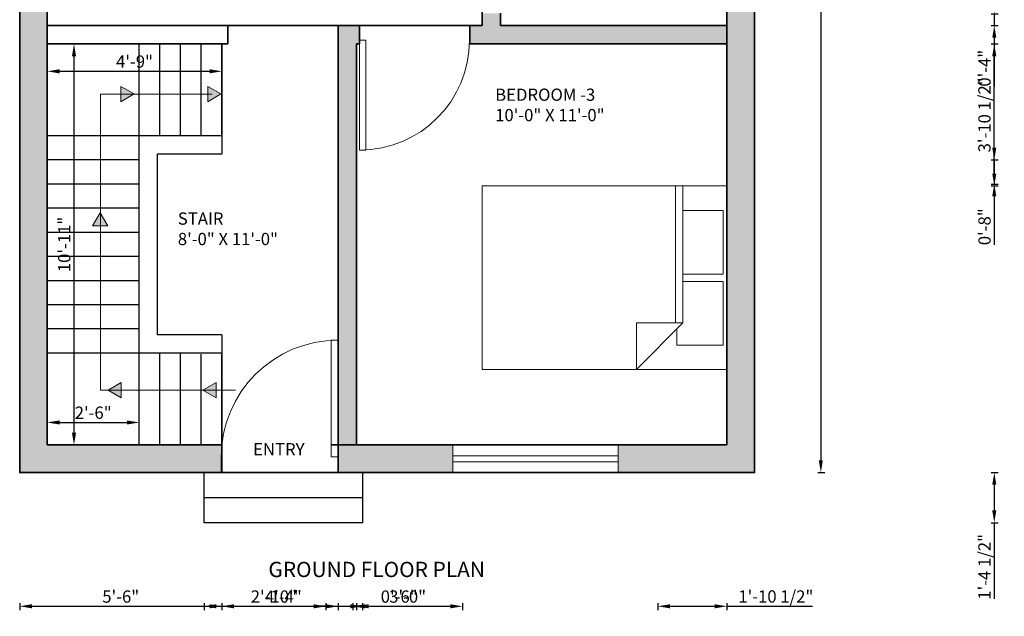
# Model space of a CAD drawing. Units: inches. Extents: x -35 to 322, y -513 to 50.
# Tile 1 of 3: x 1 to 322, y -513 to -318. Entities that reach past the tile are written whole.
import ezdxf

# ---------------------------------------------------------------- set-up
doc = ezdxf.new("R2010")
doc.units = ezdxf.units.IN
for name, color, linetype, lineweight in [('A-ANNO-DIMS', 2, 'Continuous', 18), ('A-ANNO-SYMB', 7, 'Continuous', 18), ('A-ANNO-TEXT', 7, 'Continuous', 25), ('A-AREA-IDEN', 7, 'Continuous', 18), ('A-DOOR', 4, 'Continuous', 18), ('A-FLOR-STRS', 7, 'Continuous', 25), ('A-FURN', 8, 'Continuous', 18), ('A-GLAZ', 6, 'Continuous', 18), ('A-WALL', 7, 'Continuous', 35), ('A-WALL-PATT', 251, 'Continuous', 13)]:
    doc.layers.add(name, color=color, linetype=linetype, lineweight=lineweight)
doc.styles.get("Standard").update_dxf_attribs({"font": 'arial.ttf'})
doc.dimstyles.new('ISO-25', dxfattribs={"dimtxt": 4, "dimasz": 4, "dimexe": 1.25, "dimexo": 0.625, "dimtad": 1, "dimlunit": 3, "dimtxsty": 'Standard', "dimcen": 2.5, "dimadec": 0, "dimazin": 0, "dimtfac": 1, "dimtmove": 0, "dimatfit": 3, "dimfxl": 1, "dimfxlon": 1, "dimarcsym": 0})

# ---------------------------------------------------------------- blocks, each defined once
blk = doc.blocks.new('*U4')
for p, q in [((0, 0), (0, -100)), ((750, 0), (750, -100))]:
    blk.add_line(p, q)
blk.add_lwpolyline([(0, 0), (0, 750), (43.75, 750), (43.75, 0)], close=True)
blk.add_arc((0, 0), 750, 0, 90)
blk = doc.blocks.new('Bed - Queen')
for p, q in [((0, -80.00003), (0, 0)), ((0, 0), (59.99999, 0)), ((59.99999, 0), (59.99999, -80.00003)), ((7.99999, -1.2), (28.79998, -1.2)), ((7.99999, -14.4), (7.99999, -1.2)), ((28.79998, -1.2), (28.79998, -14.4)), ((31.19999, -1.2), (51.99999, -1.2)), ((31.19999, -14.4), (31.19999, -1.2)), ((51.99999, -1.2), (51.99999, -16.4)), ((0, -14.4), (44.8, -14.4)), ((59.99999, -29.6), (44.8, -14.4)), ((44.8, -14.4), (44.8, -29.6)), ((44.8, -16.8), (0, -16.8)), ((51.99999, -16.4), (46.79936, -16.4)), ((44.8, -29.6), (59.99999, -29.6)), ((59.99999, -80.00003), (0, -80.00003))]:
    blk.add_line(p, q)
blk = doc.blocks.new('*D9')
at = {"layer": 'A-ANNO-DIMS', "color": 0, "lineweight": -2, "transparency": 16777216}
for p, q in [((9.64, -450.66), (9.64, -448.41)), ((13.64, -449.66), (35.64, -449.66)), ((39.64, -450.66), (39.64, -448.41))]:
    blk.add_line(p, q, dxfattribs=at)
at = {"layer": 'A-ANNO-DIMS', "color": 0, "transparency": 16777216}
for points in [[(13.64, -448.99), (13.64, -450.32), (9.64, -449.66)], [(35.64, -448.99), (35.64, -450.32), (39.64, -449.66)]]:
    blk.add_solid(points, dxfattribs=at)
at = {"layer": 'Defpoints', "color": 0, "transparency": 16777216}
for p in [(39.64, -449.66), (39.64, -455.32), (9.64, -457.01)]:
    blk.add_point(p, dxfattribs=at)
at = {"layer": 'A-ANNO-DIMS', "color": 0, "transparency": 16777216, "insert": (24.64, -446.99), "char_height": 4, "attachment_point": 5}
blk.add_mtext('2\'-6"', dxfattribs=at)
blk = doc.blocks.new('*D10')
at = {"layer": 'A-ANNO-DIMS', "color": 0, "lineweight": -2, "transparency": 16777216}
for p, q in [((17.38, -326.01), (19.63, -326.01)), ((18.38, -453.01), (18.38, -330.01)), ((17.38, -457.01), (19.63, -457.01))]:
    blk.add_line(p, q, dxfattribs=at)
at = {"layer": 'A-ANNO-DIMS', "color": 0, "transparency": 16777216}
for points in [[(17.71, -330.01), (19.04, -330.01), (18.38, -326.01)], [(17.71, -453.01), (19.04, -453.01), (18.38, -457.01)]]:
    blk.add_solid(points, dxfattribs=at)
at = {"layer": 'Defpoints', "color": 0, "transparency": 16777216}
for p in [(9.64, -326.01), (18.38, -326.01), (9.64, -457.01)]:
    blk.add_point(p, dxfattribs=at)
at = {"layer": 'A-ANNO-DIMS', "color": 0, "transparency": 16777216, "insert": (15.71, -391.51), "char_height": 4, "attachment_point": 5, "rotation": 90}
blk.add_mtext('10\'-11"', dxfattribs=at)
blk = doc.blocks.new('*D11')
at = {"layer": 'A-ANNO-DIMS', "color": 0, "lineweight": -2, "transparency": 16777216}
for p, q in [((9.64, -333.96), (9.64, -336.21)), ((66.64, -333.96), (66.64, -336.21)), ((13.64, -334.96), (62.64, -334.96))]:
    blk.add_line(p, q, dxfattribs=at)
at = {"layer": 'A-ANNO-DIMS', "color": 0, "transparency": 16777216}
for points in [[(13.64, -334.29), (13.64, -335.62), (9.64, -334.96)], [(62.64, -334.29), (62.64, -335.62), (66.64, -334.96)]]:
    blk.add_solid(points, dxfattribs=at)
at = {"layer": 'Defpoints', "color": 0, "transparency": 16777216}
for p in [(9.64, -326.01), (66.64, -326.01), (66.64, -334.96)]:
    blk.add_point(p, dxfattribs=at)
at = {"layer": 'A-ANNO-DIMS', "color": 0, "transparency": 16777216, "insert": (38.14, -332.29), "char_height": 4, "attachment_point": 5}
blk.add_mtext('4\'-9"', dxfattribs=at)
blk = doc.blocks.new('*D13')
at = {"layer": 'A-ANNO-DIMS', "color": 0, "lineweight": -2, "transparency": 16777216}
for p, q in [((261.29, 13.99), (263.54, 13.99)), ((262.29, 9.99), (262.29, -462.01)), ((261.29, -466.01), (263.54, -466.01))]:
    blk.add_line(p, q, dxfattribs=at)
at = {"layer": 'A-ANNO-DIMS', "color": 0, "transparency": 16777216}
for points in [[(261.62, 9.99), (262.95, 9.99), (262.29, 13.99)], [(261.62, -462.01), (262.95, -462.01), (262.29, -466.01)]]:
    blk.add_solid(points, dxfattribs=at)
at = {"layer": 'Defpoints', "color": 0, "transparency": 16777216}
for p in [(239.43, 13.99), (240.64, -466.01), (262.29, -466.01)]:
    blk.add_point(p, dxfattribs=at)
at = {"layer": 'A-ANNO-DIMS', "color": 0, "transparency": 16777216, "insert": (259.62, -226.01), "char_height": 4, "attachment_point": 5, "rotation": 90}
blk.add_mtext("40'", dxfattribs=at)
blk = doc.blocks.new('STAIR-DIRECTION-ARROW')
h = blk.add_hatch(color=256)
h.dxf.hatch_style = 1
h.paths.add_polyline_path([(0, 2.47), (4.31, 0), (4.31, 5)])
blk.add_lwpolyline([(4.31, 0), (4.31, 5), (0, 2.47)], close=True)
blk = doc.blocks.new('*D26')
at = {"layer": 'A-ANNO-DIMS', "color": 0, "lineweight": -2, "transparency": 16777216}
for p, q in [((100.64, -509.7), (96.64, -509.7)), ((104.64, -508.7), (104.64, -510.95)), ((104.64, -509.7), (110.64, -509.7)), ((110.64, -508.7), (110.64, -510.95)), ((114.64, -509.7), (130.52, -509.7))]:
    blk.add_line(p, q, dxfattribs=at)
at = {"layer": 'A-ANNO-DIMS', "color": 0, "transparency": 16777216}
for points in [[(100.64, -509.04), (100.64, -510.37), (104.64, -509.7)], [(114.64, -509.04), (114.64, -510.37), (110.64, -509.7)]]:
    blk.add_solid(points, dxfattribs=at)
at = {"layer": 'Defpoints', "color": 0, "transparency": 16777216}
for p in [(104.64, -77.01), (110.64, -83.01), (110.64, -509.7)]:
    blk.add_point(p, dxfattribs=at)
at = {"layer": 'A-ANNO-DIMS', "color": 0, "transparency": 16777216, "insert": (124.58, -507.04), "char_height": 4, "attachment_point": 5}
blk.add_mtext('0\'-6"', dxfattribs=at)
blk = doc.blocks.new('*D27')
at = {"layer": 'A-ANNO-DIMS', "color": 0, "lineweight": -2, "transparency": 16777216}
for p, q in [((60.84, -508.7), (60.84, -510.95)), ((64.84, -509.7), (108.62, -509.7)), ((112.62, -508.7), (112.62, -510.95))]:
    blk.add_line(p, q, dxfattribs=at)
at = {"layer": 'A-ANNO-DIMS', "color": 0, "transparency": 16777216}
for points in [[(64.84, -509.04), (64.84, -510.37), (60.84, -509.7)], [(108.62, -509.04), (108.62, -510.37), (112.62, -509.7)]]:
    blk.add_solid(points, dxfattribs=at)
at = {"layer": 'Defpoints', "color": 0, "transparency": 16777216}
for p in [(60.84, -482.4), (112.62, -482.4), (112.62, -509.7)]:
    blk.add_point(p, dxfattribs=at)
at = {"layer": 'A-ANNO-DIMS', "color": 0, "transparency": 16777216, "insert": (86.73, -507.08), "char_height": 4, "attachment_point": 5}
blk.add_mtext('4\'-4"', dxfattribs=at)
blk = doc.blocks.new('*D28')
at = {"layer": 'A-ANNO-DIMS', "color": 0, "lineweight": -2, "transparency": 16777216}
for p, q in [((317.94, -466.01), (320.19, -466.01)), ((318.94, -470.01), (318.94, -478.4)), ((317.94, -482.4), (320.19, -482.4)), ((318.94, -482.4), (318.94, -507.23))]:
    blk.add_line(p, q, dxfattribs=at)
at = {"layer": 'A-ANNO-DIMS', "color": 0, "transparency": 16777216}
for points in [[(318.27, -470.01), (319.6, -470.01), (318.94, -466.01)], [(318.27, -478.4), (319.6, -478.4), (318.94, -482.4)]]:
    blk.add_solid(points, dxfattribs=at)
at = {"layer": 'Defpoints', "color": 0, "transparency": 16777216}
for p in [(112.62, -466.01), (112.62, -482.4), (318.94, -482.4)]:
    blk.add_point(p, dxfattribs=at)
at = {"layer": 'A-ANNO-DIMS', "color": 0, "transparency": 16777216, "insert": (316.24, -496.82), "char_height": 4, "attachment_point": 5, "rotation": 90}
blk.add_mtext('1\'-4 1/2"', dxfattribs=at)
blk = doc.blocks.new('*D29')
at = {"layer": 'A-ANNO-DIMS', "color": 0, "lineweight": -2, "transparency": 16777216}
for p, q in [((66.64, 40.29), (66.64, 42.54)), ((104.64, 40.29), (104.64, 42.54)), ((70.64, 41.29), (100.64, 41.29))]:
    blk.add_line(p, q, dxfattribs=at)
at = {"layer": 'A-ANNO-DIMS', "color": 0, "transparency": 16777216}
for points in [[(70.64, 41.95), (70.64, 40.62), (66.64, 41.29)], [(100.64, 41.95), (100.64, 40.62), (104.64, 41.29)]]:
    blk.add_solid(points, dxfattribs=at)
at = {"layer": 'Defpoints', "color": 0, "transparency": 16777216}
for p in [(104.64, 41.29), (66.64, -466.01), (104.64, -466.01)]:
    blk.add_point(p, dxfattribs=at)
at = {"layer": 'A-ANNO-DIMS', "color": 0, "transparency": 16777216, "insert": (85.64, 43.96), "char_height": 4, "attachment_point": 5}
blk.add_mtext('3\'-2"', dxfattribs=at)
blk = doc.blocks.new('*D30')
at = {"layer": 'A-ANNO-DIMS', "color": 0, "lineweight": -2, "transparency": 16777216}
for p, q in [((0.64, -508.7), (0.64, -510.95)), ((4.64, -509.7), (62.64, -509.7)), ((66.64, -508.7), (66.64, -510.95))]:
    blk.add_line(p, q, dxfattribs=at)
at = {"layer": 'A-ANNO-DIMS', "color": 0, "transparency": 16777216}
for points in [[(4.64, -509.04), (4.64, -510.37), (0.64, -509.7)], [(62.64, -509.04), (62.64, -510.37), (66.64, -509.7)]]:
    blk.add_solid(points, dxfattribs=at)
at = {"layer": 'Defpoints', "color": 0, "transparency": 16777216}
for p in [(0.64, -466.01), (66.64, -466.01), (66.64, -509.7)]:
    blk.add_point(p, dxfattribs=at)
at = {"layer": 'A-ANNO-DIMS', "color": 0, "transparency": 16777216, "insert": (33.64, -507.04), "char_height": 4, "attachment_point": 5}
blk.add_mtext('5\'-6"', dxfattribs=at)
blk = doc.blocks.new('*D42')
at = {"layer": 'A-ANNO-DIMS', "color": 0, "lineweight": -2, "transparency": 16777216}
for p, q in [((196.08, 40.29), (196.08, 42.54)), ((231.64, 40.29), (231.64, 42.54)), ((200.08, 41.29), (227.64, 41.29))]:
    blk.add_line(p, q, dxfattribs=at)
at = {"layer": 'A-ANNO-DIMS', "color": 0, "transparency": 16777216}
for points in [[(200.08, 41.95), (200.08, 40.62), (196.08, 41.29)], [(227.64, 41.95), (227.64, 40.62), (231.64, 41.29)]]:
    blk.add_solid(points, dxfattribs=at)
at = {"layer": 'Defpoints', "color": 0, "transparency": 16777216}
for p in [(231.64, 41.29), (196.08, -457.01), (231.64, -457.01)]:
    blk.add_point(p, dxfattribs=at)
at = {"layer": 'A-ANNO-DIMS', "color": 0, "transparency": 16777216, "insert": (213.86, 43.98), "char_height": 4, "attachment_point": 5}
blk.add_mtext('2\'-11 1/2"', dxfattribs=at)
blk = doc.blocks.new('*D43')
at = {"layer": 'A-ANNO-DIMS', "color": 0, "lineweight": -2, "transparency": 16777216}
for p, q in [((66.64, -508.7), (66.64, -510.95)), ((70.64, -509.7), (96.64, -509.7)), ((100.64, -508.7), (100.64, -510.95))]:
    blk.add_line(p, q, dxfattribs=at)
at = {"layer": 'A-ANNO-DIMS', "color": 0, "transparency": 16777216}
for points in [[(70.64, -509.04), (70.64, -510.37), (66.64, -509.7)], [(96.64, -509.04), (96.64, -510.37), (100.64, -509.7)]]:
    blk.add_solid(points, dxfattribs=at)
at = {"layer": 'Defpoints', "color": 0, "transparency": 16777216}
for p in [(66.64, -83.01), (100.64, -83.01), (100.64, -509.7)]:
    blk.add_point(p, dxfattribs=at)
at = {"layer": 'A-ANNO-DIMS', "color": 0, "transparency": 16777216, "insert": (83.64, -507.04), "char_height": 4, "attachment_point": 5}
blk.add_mtext('2\'-10"', dxfattribs=at)
blk = doc.blocks.new('*D48')
at = {"layer": 'A-ANNO-DIMS', "color": 0, "lineweight": -2, "transparency": 16777216}
for p, q in [((109.42, -508.7), (109.42, -510.95)), ((113.42, -509.7), (141.25, -509.7)), ((145.25, -508.7), (145.25, -510.95))]:
    blk.add_line(p, q, dxfattribs=at)
at = {"layer": 'A-ANNO-DIMS', "color": 0, "transparency": 16777216}
for points in [[(113.42, -509.04), (113.42, -510.37), (109.42, -509.7)], [(141.25, -509.04), (141.25, -510.37), (145.25, -509.7)]]:
    blk.add_solid(points, dxfattribs=at)
at = {"layer": 'Defpoints', "color": 0, "transparency": 16777216}
for p in [(109.42, -131.05), (145.25, -131.34), (145.25, -509.7)]:
    blk.add_point(p, dxfattribs=at)
at = {"layer": 'A-ANNO-DIMS', "color": 0, "transparency": 16777216, "insert": (127.34, -507.04), "char_height": 4, "attachment_point": 5}
blk.add_mtext('3\'-0"', dxfattribs=at)
blk = doc.blocks.new('*D50')
at = {"layer": 'A-ANNO-DIMS', "color": 0, "lineweight": -2, "transparency": 16777216}
for p, q in [((111.64, 40.29), (111.64, 42.54)), ((147.64, 40.29), (147.64, 42.54)), ((115.64, 41.29), (143.64, 41.29))]:
    blk.add_line(p, q, dxfattribs=at)
at = {"layer": 'A-ANNO-DIMS', "color": 0, "transparency": 16777216}
for points in [[(115.64, 41.95), (115.64, 40.62), (111.64, 41.29)], [(143.64, 41.95), (143.64, 40.62), (147.64, 41.29)]]:
    blk.add_solid(points, dxfattribs=at)
at = {"layer": 'Defpoints', "color": 0, "transparency": 16777216}
for p in [(147.64, 41.29), (111.64, -320.01), (147.64, -320.01)]:
    blk.add_point(p, dxfattribs=at)
at = {"layer": 'A-ANNO-DIMS', "color": 0, "transparency": 16777216, "insert": (129.64, 43.96), "char_height": 4, "attachment_point": 5}
blk.add_mtext('3\'-0"', dxfattribs=at)
blk = doc.blocks.new('*D53')
at = {"layer": 'A-ANNO-DIMS', "color": 0, "lineweight": -2, "transparency": 16777216}
for p, q in [((318.94, -312.18), (318.94, -308.18)), ((317.94, -316.18), (320.19, -316.18)), ((318.94, -316.18), (318.94, -320.01)), ((317.94, -320.01), (320.19, -320.01)), ((318.94, -324.01), (318.94, -339.9))]:
    blk.add_line(p, q, dxfattribs=at)
at = {"layer": 'A-ANNO-DIMS', "color": 0, "transparency": 16777216}
for points in [[(318.27, -312.18), (319.6, -312.18), (318.94, -316.18)], [(318.27, -324.01), (319.6, -324.01), (318.94, -320.01)]]:
    blk.add_solid(points, dxfattribs=at)
at = {"layer": 'Defpoints', "color": 0, "transparency": 16777216}
for p in [(231.64, -316.18), (231.64, -320.01), (318.94, -320.01)]:
    blk.add_point(p, dxfattribs=at)
at = {"layer": 'A-ANNO-DIMS', "color": 0, "transparency": 16777216, "insert": (316.27, -333.95), "char_height": 4, "attachment_point": 5, "rotation": 90}
blk.add_mtext('0\'-4"', dxfattribs=at)
blk = doc.blocks.new('*D54')
at = {"layer": 'A-ANNO-DIMS', "color": 0, "lineweight": -2, "transparency": 16777216}
for p, q in [((209.06, -508.7), (209.06, -510.95)), ((213.06, -509.7), (227.64, -509.7)), ((231.64, -508.7), (231.64, -510.95)), ((231.64, -509.7), (259.57, -509.7))]:
    blk.add_line(p, q, dxfattribs=at)
at = {"layer": 'A-ANNO-DIMS', "color": 0, "transparency": 16777216}
for points in [[(213.06, -509.04), (213.06, -510.37), (209.06, -509.7)], [(227.64, -509.04), (227.64, -510.37), (231.64, -509.7)]]:
    blk.add_solid(points, dxfattribs=at)
at = {"layer": 'Defpoints', "color": 0, "transparency": 16777216}
for p in [(209.06, 4.99), (231.64, 4.99), (231.64, -509.7)]:
    blk.add_point(p, dxfattribs=at)
at = {"layer": 'A-ANNO-DIMS', "color": 0, "transparency": 16777216, "insert": (247.6, -507.01), "char_height": 4, "attachment_point": 5}
blk.add_mtext('1\'-10 1/2"', dxfattribs=at)
blk = doc.blocks.new('*D56')
at = {"layer": 'A-ANNO-DIMS', "color": 0, "lineweight": -2, "transparency": 16777216}
for p, q in [((317.94, -326.01), (320.19, -326.01)), ((318.94, -368.37), (318.94, -330.01)), ((317.94, -372.37), (320.19, -372.37))]:
    blk.add_line(p, q, dxfattribs=at)
at = {"layer": 'A-ANNO-DIMS', "color": 0, "transparency": 16777216}
for points in [[(318.27, -330.01), (319.6, -330.01), (318.94, -326.01)], [(318.27, -368.37), (319.6, -368.37), (318.94, -372.37)]]:
    blk.add_solid(points, dxfattribs=at)
at = {"layer": 'Defpoints', "color": 0, "transparency": 16777216}
for p in [(147.64, -326.01), (318.94, -326.01), (151.64, -372.37)]:
    blk.add_point(p, dxfattribs=at)
at = {"layer": 'A-ANNO-DIMS', "color": 0, "transparency": 16777216, "insert": (316.24, -349.19), "char_height": 4, "attachment_point": 5, "rotation": 90}
blk.add_mtext('3\'-10 1/2"', dxfattribs=at)
blk = doc.blocks.new('*D61')
at = {"layer": 'A-ANNO-DIMS', "color": 0, "lineweight": -2, "transparency": 16777216}
for p, q in [((39.64, 40.29), (39.64, 42.54)), ((46.39, 40.29), (46.39, 42.54)), ((35.64, 41.29), (31.64, 41.29)), ((39.64, 41.29), (46.39, 41.29)), ((50.39, 41.29), (66.27, 41.29))]:
    blk.add_line(p, q, dxfattribs=at)
at = {"layer": 'A-ANNO-DIMS', "color": 0, "transparency": 16777216}
for points in [[(35.64, 41.95), (35.64, 40.62), (39.64, 41.29)], [(50.39, 41.95), (50.39, 40.62), (46.39, 41.29)]]:
    blk.add_solid(points, dxfattribs=at)
at = {"layer": 'Defpoints', "color": 0, "transparency": 16777216}
for p in [(46.39, 41.29), (39.64, -326.01), (46.39, -326.01)]:
    blk.add_point(p, dxfattribs=at)
at = {"layer": 'A-ANNO-DIMS', "color": 0, "transparency": 16777216, "insert": (60.33, 43.95), "char_height": 4, "attachment_point": 5}
blk.add_mtext('0\'-7"', dxfattribs=at)
blk = doc.blocks.new('*D62')
at = {"layer": 'A-ANNO-DIMS', "color": 0, "lineweight": -2, "transparency": 16777216}
for p, q in [((318.94, -359.9), (318.94, -355.9)), ((317.94, -363.9), (320.19, -363.9)), ((318.94, -363.9), (318.94, -371.79)), ((317.94, -371.79), (320.19, -371.79)), ((318.94, -375.79), (318.94, -391.67))]:
    blk.add_line(p, q, dxfattribs=at)
at = {"layer": 'A-ANNO-DIMS', "color": 0, "transparency": 16777216}
for points in [[(318.27, -359.9), (319.6, -359.9), (318.94, -363.9)], [(318.27, -375.79), (319.6, -375.79), (318.94, -371.79)]]:
    blk.add_solid(points, dxfattribs=at)
at = {"layer": 'Defpoints', "color": 0, "transparency": 16777216}
for p in [(39.64, -363.9), (39.64, -371.79), (318.94, -371.79)]:
    blk.add_point(p, dxfattribs=at)
at = {"layer": 'A-ANNO-DIMS', "color": 0, "transparency": 16777216, "insert": (316.27, -385.73), "char_height": 4, "attachment_point": 5, "rotation": 90}
blk.add_mtext('0\'-8"', dxfattribs=at)

msp = doc.modelspace()

# ---------------------------------------------------------------- hatches: boundary and pattern name
at = {"layer": 'A-WALL-PATT'}
h = msp.add_hatch(color=256, dxfattribs=at)
h.dxf.hatch_style = 1
h.paths.add_polyline_path([(63.099, 13.987), (0.637, 13.987), (0.637, -26.079), (9.637, -26.079), (9.637, 4.987), (63.099, 4.987)])
h.paths.add_polyline_path([(9.637, -107.554), (0.637, -107.554), (0.637, -205.04), (9.637, -205.04)])
h.paths.add_polyline_path([(9.637, -60.079), (0.637, -60.079), (0.637, -89.554), (9.637, -89.554)])
h.paths.add_polyline_path([(9.637, -259.04), (0.637, -259.04), (0.637, -466.013), (66.468, -466.013), (66.468, -460.924, -0.0235925), (66.637, -457.328), (66.637, -457.013), (9.637, -457.013), (9.637, -326.013)])
h.paths.add_polyline_path([(142.082, -457.013), (104.637, -457.013), (104.637, -460.924), (104.637, -466.013), (142.082, -466.013)])
h.paths.add_polyline_path([(240.637, -224.716), (231.637, -224.716), (231.637, -274.623), (240.637, -274.623)])
h.paths.add_polyline_path([(69.474, -113.132), (98.939, -113.132), (98.939, -98.154), (69.474, -98.154)], flags=9)
h.paths.add_polyline_path([(38.843, -240.589), (73.258, -240.589), (73.258, -225.663), (38.843, -225.663)], flags=9)
h.paths.add_polyline_path([(51.03, -393.995), (85.248, -393.995), (85.248, -379.069), (51.03, -379.069)], flags=9)
h.paths.add_polyline_path([(75.428, -462.589), (96.367, -462.589), (96.367, -454.346), (75.428, -454.346)], flags=9)
h.paths.add_polyline_path([(154.313, -353.536), (191.907, -353.536), (191.907, -338.61), (154.313, -338.61)], flags=9)
h.paths.add_polyline_path([(177.411, -284.106), (208.497, -284.106), (208.497, -269.18), (177.411, -269.18)], flags=9)
h.paths.add_polyline_path([(152.205, -160.654), (189.798, -160.654), (189.798, -145.728), (152.205, -145.728)], flags=9)
h.paths.add_polyline_path([(150.351, -98.334), (187.945, -98.334), (187.945, -83.408), (150.351, -83.408)], flags=9)
h.paths.add_polyline_path([(15.293, -117.178), (49.667, -117.178), (49.667, -102.252), (15.293, -102.252)], flags=9)
h.paths.add_polyline_path([(40.377, -44.483), (77.823, -44.483), (77.823, -29.557), (40.377, -29.557)], flags=9)
h.paths.add_polyline_path([(31.67, -336.447), (44.796, -336.447), (44.796, -328.204), (31.67, -328.204)], flags=25)
h = msp.add_hatch(color=256, dxfattribs=at)
h.dxf.hatch_style = 1
h.paths.add_polyline_path([(110.637, 4.987), (104.637, 4.987), (104.637, -77.013), (100.637, -77.013), (100.637, -78.48), (100.637, -83.013), (104.637, -83.013), (110.637, -83.013)])
h.paths.add_polyline_path([(231.637, -121.013), (110.637, -121.013), (110.637, -117.013), (109.17, -117.013), (104.637, -117.013), (104.637, -131.013), (110.637, -131.013), (110.637, -127.013), (231.637, -127.013)])
h.paths.add_polyline_path([(15.293, -117.178), (49.667, -117.178), (49.667, -102.252), (15.293, -102.252)], flags=9)
h.paths.add_polyline_path([(69.474, -113.132), (98.939, -113.132), (98.939, -98.154), (69.474, -98.154)], flags=9)
h.paths.add_polyline_path([(38.843, -240.589), (73.258, -240.589), (73.258, -225.663), (38.843, -225.663)], flags=9)
h.paths.add_polyline_path([(51.03, -393.995), (85.248, -393.995), (85.248, -379.069), (51.03, -379.069)], flags=9)
h.paths.add_polyline_path([(75.428, -462.589), (96.367, -462.589), (96.367, -454.346), (75.428, -454.346)], flags=9)
h.paths.add_polyline_path([(154.313, -353.536), (191.907, -353.536), (191.907, -338.61), (154.313, -338.61)], flags=9)
h.paths.add_polyline_path([(177.411, -284.106), (208.497, -284.106), (208.497, -269.18), (177.411, -269.18)], flags=9)
h.paths.add_polyline_path([(152.205, -160.654), (189.798, -160.654), (189.798, -145.728), (152.205, -145.728)], flags=9)
h.paths.add_polyline_path([(150.351, -98.334), (187.945, -98.334), (187.945, -83.408), (150.351, -83.408)], flags=9)
h.paths.add_polyline_path([(40.377, -44.483), (77.823, -44.483), (77.823, -29.557), (40.377, -29.557)], flags=9)
h = msp.add_hatch(color=256, dxfattribs=at)
h.dxf.hatch_style = 1
h.paths.add_polyline_path([(110.637, -326.013), (111.637, -326.013), (111.637, -324.8), (111.637, -320.013), (104.637, -320.013), (104.637, -457.013), (110.637, -457.013)])
h.paths.add_polyline_path([(231.637, -320.013), (157.637, -320.013), (157.637, -316.013), (153.631, -316.013), (151.637, -316.029), (151.637, -320.013), (147.637, -320.013), (147.637, -326.013), (151.637, -326.013), (157.637, -326.013), (231.637, -326.013)])
h.paths.add_polyline_path([(240.637, -292.623), (231.637, -292.623), (231.637, -457.013), (196.082, -457.013), (196.082, -466.013), (240.637, -466.013)])
h.paths.add_polyline_path([(15.293, -117.178), (49.667, -117.178), (49.667, -102.252), (15.293, -102.252)], flags=9)
h.paths.add_polyline_path([(69.474, -113.132), (98.939, -113.132), (98.939, -98.154), (69.474, -98.154)], flags=9)
h.paths.add_polyline_path([(38.843, -240.589), (73.258, -240.589), (73.258, -225.663), (38.843, -225.663)], flags=9)
h.paths.add_polyline_path([(51.03, -393.995), (85.248, -393.995), (85.248, -379.069), (51.03, -379.069)], flags=9)
h.paths.add_polyline_path([(75.428, -462.589), (96.367, -462.589), (96.367, -454.346), (75.428, -454.346)], flags=9)
h.paths.add_polyline_path([(154.313, -353.536), (191.907, -353.536), (191.907, -338.61), (154.313, -338.61)], flags=9)
h.paths.add_polyline_path([(152.205, -160.654), (189.798, -160.654), (189.798, -145.728), (152.205, -145.728)], flags=9)
h.paths.add_polyline_path([(150.351, -98.334), (187.945, -98.334), (187.945, -83.408), (150.351, -83.408)], flags=9)
h.paths.add_polyline_path([(40.377, -44.483), (77.823, -44.483), (77.823, -29.557), (40.377, -29.557)], flags=9)

# ---------------------------------------------------------------- linework, layer by layer
at = {"layer": 'A-ANNO-SYMB'}
for p, q in [((27.019, -439.101), (27.019, -342.386)), ((27.019, -342.386), (63.481, -342.386)), ((71.075, -439.101), (27.019, -439.101))]:
    msp.add_line(p, q, dxfattribs=at)
at = {"layer": 'A-FLOR-STRS'}
for p, q in [((39.637, -356.013), (39.637, -326.013)), ((46.387, -356.013), (46.387, -326.013)), ((53.137, -356.013), (53.137, -326.013)), ((59.887, -356.013), (59.887, -326.013)), ((66.637, -326.013), (66.637, -362.013)), ((66.637, -356.013), (66.637, -326.013)), ((39.637, -356.013), (9.637, -356.013)), ((66.637, -356.013), (39.637, -356.013)), ((39.637, -362.013), (39.637, -356.013)), ((39.637, -421.013), (39.637, -362.013)), ((66.637, -362.013), (45.637, -362.013)), ((45.637, -421.013), (45.637, -362.013)), ((39.637, -363.902), (9.637, -363.902)), ((39.637, -371.791), (9.637, -371.791)), ((39.637, -379.68), (9.637, -379.68)), ((39.637, -387.569), (9.637, -387.569)), ((39.637, -395.458), (9.637, -395.458)), ((39.637, -403.346), (9.637, -403.346)), ((39.637, -411.235), (9.637, -411.235)), ((39.637, -419.124), (9.637, -419.124)), ((39.637, -427.013), (39.637, -421.013)), ((66.637, -421.013), (45.637, -421.013)), ((66.637, -421.013), (66.637, -457.013)), ((39.637, -427.013), (9.637, -427.013)), ((39.637, -427.013), (9.637, -427.013)), ((39.637, -457.013), (39.637, -427.013)), ((66.637, -427.013), (39.637, -427.013)), ((46.387, -457.013), (46.387, -427.118)), ((53.137, -457.013), (53.137, -427.224)), ((59.887, -457.013), (59.887, -427.329)), ((66.637, -457.013), (66.637, -427.435)), ((60.841, -474.209), (112.62, -474.209))]:
    msp.add_line(p, q, dxfattribs=at)
msp.add_lwpolyline([(60.841, -466.013), (112.62, -466.013), (112.62, -482.404), (60.841, -482.404)], close=True, dxfattribs=at)
at = {"layer": 'A-GLAZ'}
for p, q in [((196.082, -460.513), (142.082, -460.513)), ((196.082, -462.513), (142.082, -462.513))]:
    msp.add_line(p, q, dxfattribs=at)
msp.add_lwpolyline([(196.082, -457.013), (196.082, -466.013), (142.082, -466.013), (142.082, -457.013)], close=True, dxfattribs=at)
at = {"layer": 'A-WALL'}
for p, q in [((9.637, -326.013), (9.637, 4.987)), ((231.637, 4.987), (231.637, -457.013)), ((151.637, -265.013), (151.637, -320.013)), ((157.637, -316.013), (157.637, -320.013)), ((104.637, -320.013), (9.637, -320.013)), ((68.637, -326.013), (68.637, -320.013)), ((104.637, -457.013), (104.637, -320.013)), ((151.637, -320.013), (104.637, -320.013)), ((111.637, -320.013), (111.637, -326.013)), ((147.637, -320.013), (147.637, -326.013)), ((157.637, -320.013), (231.637, -320.013)), ((9.637, -457.013), (9.637, -326.013)), ((68.637, -326.013), (9.637, -326.013)), ((110.637, -457.013), (110.637, -326.013)), ((111.637, -326.013), (110.637, -326.013)), ((151.637, -326.013), (147.637, -326.013)), ((157.637, -326.013), (151.637, -326.013)), ((157.637, -326.013), (231.637, -326.013)), ((66.669, -457.013), (9.637, -457.013)), ((66.637, -457.013), (66.637, -466.013)), ((231.637, -457.013), (102.411, -457.013)), ((104.637, -457.013), (104.637, -466.013))]:
    msp.add_line(p, q, dxfattribs=at)
msp.add_lwpolyline([(0.637, 13.987), (240.637, 13.987), (240.637, -466.013), (0.637, -466.013)], close=True, dxfattribs=at)

# ---------------------------------------------------------------- block references
at = {"layer": 'A-ANNO-SYMB'}
for p, rotation in [((38.03, -339.897), 180), ((66.354, -339.897), 180), ((24.45, -381.153), 270.000000000001)]:
    msp.add_blockref('STAIR-DIRECTION-ARROW', p, dxfattribs=dict(at, rotation=rotation))
for p in [(29.499, -441.601), (60.468, -441.601)]:
    msp.add_blockref('STAIR-DIRECTION-ARROW', p, dxfattribs=at)
at = {"layer": 'A-DOOR', "xscale": -0.0478695843838057, "yscale": 0.0478695843838057, "zscale": 0.0478695843838057, "rotation": 180}
msp.add_blockref('*U4', (111.637, -324.8), dxfattribs=at)
at = {"layer": 'A-DOOR', "xscale": -0.0508930330465815, "yscale": 0.0508930330465815, "zscale": 0.0508930330465815}
msp.add_blockref('*U4', (104.637, -460.924), dxfattribs=at)
at = {"layer": 'A-FURN', "rotation": 270}
msp.add_blockref('Bed - Queen', (231.637, -372.367), dxfattribs=at)

# ---------------------------------------------------------------- texts
at = {"layer": 'A-ANNO-TEXT', "insert": (81.873, -495.17), "char_height": 5, "attachment_point": 1}
msp.add_mtext_dynamic_manual_height_columns('GROUND FLOOR PLAN', width=112.78265, gutter_width=12.5, heights=[0], dxfattribs=at)
at = {"layer": 'A-AREA-IDEN', "char_height": 4, "attachment_point": 1}
for s, width, insert in [('BEDROOM -3\\P10\'-0" X 11\'-0"', 61.18238, (155.922, -340.598)), ('STAIR\\P8\'-0" X 11\'-0"', 39.79833, (52.281, -381.06)), ('ENTRY', 21.21407, (76.87, -456.405))]:
    msp.add_mtext_dynamic_manual_height_columns(s, width=width, gutter_width=12.5, heights=[0], dxfattribs=dict(at, insert=insert))

# ---------------------------------------------------------------- dimensions: what is measured, and where the dimension line sits
at = {"layer": 'A-ANNO-DIMS'}
for base, p1, p2, override, picture, middle in [((231.637, 41.287), (196.082, -457.013), (231.637, -457.013), {"dimdec": 1, "dimlfac": 1, "dimrnd": 0, "dimzin": 1, "dimdsep": 46, "dimlunit": 4, "dimfrac": 2}, '*D42', (213.86, 43.98)), ((46.387441, 41.286907), (39.637441, -326.013093), (46.387441, -326.013093), {"dimdec": 1, "dimlfac": 1, "dimrnd": 0, "dimzin": 1, "dimdsep": 46, "dimlunit": 4, "dimfrac": 2}, '*D61', (60.328948503, 43.954198951)), ((104.637, 41.287), (66.637, -466.013), (104.637, -466.013), {"dimdec": 1, "dimlfac": 1, "dimrnd": 0, "dimzin": 1, "dimdsep": 46, "dimlunit": 4, "dimfrac": 2}, '*D29', (85.637, 43.956)), ((147.637, 41.287), (111.637, -320.013), (147.637, -320.013), {"dimdec": 1, "dimlfac": 1, "dimrnd": 0, "dimzin": 1, "dimdsep": 46, "dimlunit": 4, "dimfrac": 2}, '*D50', (129.637, 43.956)), ((231.637, -509.704), (209.063, 4.987), (231.637, 4.987), {"dimdec": 1, "dimlfac": 1, "dimrnd": 0, "dimzin": 1, "dimdsep": 46, "dimlunit": 4, "dimfrac": 2}, '*D54', (247.605, -507.011)), ((110.637, -509.704), (104.637, -77.013), (110.637, -83.013), {"dimdec": 1, "dimlfac": 1, "dimrnd": 0, "dimzin": 1, "dimdsep": 46, "dimlunit": 4, "dimfrac": 2}, '*D26', (124.579, -507.037)), ((100.637, -509.704), (66.637, -83.013), (100.637, -83.013), {"dimdec": 1, "dimlfac": 1, "dimrnd": 0, "dimzin": 1, "dimdsep": 46, "dimlunit": 4, "dimfrac": 2}, '*D43', (83.637, -507.037)), ((145.255, -509.704), (109.416, -131.052), (145.255, -131.34), {"dimdec": 1, "dimlfac": 1, "dimrnd": 0, "dimzin": 1, "dimdsep": 46, "dimlunit": 4, "dimfrac": 2}, '*D48', (127.335, -507.036)), ((66.637, -334.956), (9.637, -326.013), (66.637, -326.013), {"dimclrd": 0, "dimclre": 0, "dimclrt": 0}, '*D11', (38.137, -332.289)), ((39.637, -449.656), (9.637, -457.013), (39.637, -455.323), {"dimclrd": 0, "dimclre": 0, "dimclrt": 0}, '*D9', (24.637, -446.989)), ((66.637, -509.704), (0.637, -466.013), (66.637, -466.013), {"dimdec": 1, "dimlfac": 1, "dimrnd": 0, "dimzin": 1, "dimdsep": 46, "dimlunit": 4, "dimfrac": 2}, '*D30', (33.637, -507.037)), ((112.62, -509.704), (60.841, -482.404), (112.62, -482.404), {"dimdec": 1, "dimlfac": 1, "dimrnd": 0, "dimzin": 1, "dimdsep": 46, "dimlunit": 4, "dimfrac": 2}, '*D27', (86.731, -507.079))]:
    dim = msp.add_linear_dim(base=base, p1=p1, p2=p2, dimstyle='ISO-25', override=override, dxfattribs=at)
    dim.commit()
    dim.dimension.update_dxf_attribs({"geometry": picture, "text_midpoint": middle})
for base, p1, p2, override, picture, middle in [((262.288, -466.013), (239.425, 13.987), (240.637, -466.013), {"dimclrd": 0, "dimclre": 0, "dimclrt": 0}, '*D13', (259.621, -226.013)), ((318.937, -320.013), (231.637, -316.175), (231.637, -320.013), {"dimdec": 1, "dimlfac": 1, "dimrnd": 0, "dimzin": 1, "dimdsep": 46, "dimlunit": 4, "dimfrac": 2}, '*D53', (316.27, -333.955)), ((18.377, -326.013), (9.637, -457.013), (9.637, -326.013), {"dimclrd": 0, "dimclre": 0, "dimclrt": 0}, '*D10', (15.71, -391.513)), ((318.937, -326.013), (151.637, -372.367), (147.637, -326.013), {"dimdec": 1, "dimlfac": 1, "dimrnd": 0, "dimzin": 1, "dimdsep": 46, "dimlunit": 4, "dimfrac": 2}, '*D56', (316.243, -349.19)), ((318.937, -371.791), (39.637, -363.902), (39.637, -371.791), {"dimdec": 1, "dimlfac": 1, "dimrnd": 0, "dimzin": 1, "dimdsep": 46, "dimlunit": 4, "dimfrac": 2}, '*D62', (316.27, -385.732)), ((318.937, -482.404), (112.62, -466.013), (112.62, -482.404), {"dimdec": 1, "dimlfac": 1, "dimrnd": 0, "dimzin": 1, "dimdsep": 46, "dimlunit": 4, "dimfrac": 2}, '*D28', (316.244, -496.818))]:
    dim = msp.add_linear_dim(base=base, p1=p1, p2=p2, angle=90, dimstyle='ISO-25', override=override, dxfattribs=at)
    dim.commit()
    dim.dimension.update_dxf_attribs({"geometry": picture, "text_midpoint": middle})

doc.saveas('drawing.dxf')
